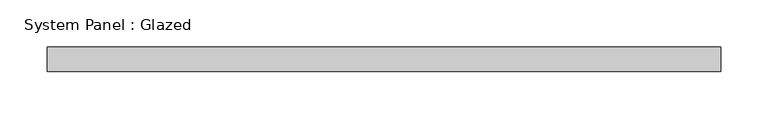
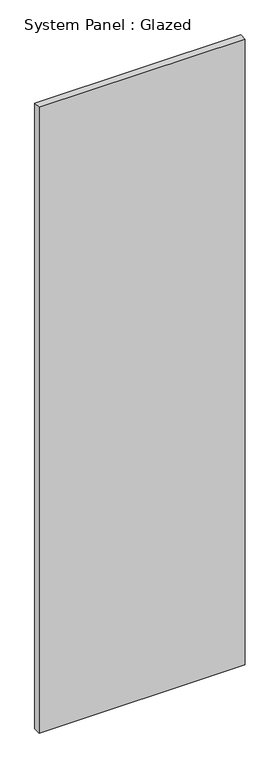
"""IFC4 building model written with IfcOpenShell, lengths in millimetres: plate geometry, System Panel : Glazed."""

from ifc_helpers import new_model, si_unit, origin, origin_with_axes, place, context, project, spatial, polyline, outline, extrude, source, transform, mapped, element, save


def system_panel_glazed_161bf594(model_context):
    return source(origin(), model_context, "Body", "SweptSolid", [
        extrude(outline(polyline([(354.5271, 19.05), (-354.5271, 19.05), (-354.5271, 44.45), (354.5271, 44.45), (354.5271, 19.05)])), origin_with_axes(), (0.0, 0.0, 1.0), 2275.4166667),
    ])


if __name__ == "__main__":
    model = new_model("IFC4")
    model_context = context("Model", 3, world=origin())
    ifc_project = project(units=[si_unit("LENGTHUNIT", "METRE", prefix="MILLI")], contexts=[model_context])
    site = spatial("IfcSite", under=ifc_project)
    building = spatial("IfcBuilding", under=site)
    placement = place(None, origin())
    system_panel_glazed_shape = system_panel_glazed_161bf594(model_context)
    element("IfcPlate", 1, ObjectType="System Panel : Glazed", at=placement, inside=building, context=model_context, shape_type="MappedRepresentation", body=[
        mapped(system_panel_glazed_shape, transform((0.0, 0.0, 0.0), x_axis=(1.0, 0.0, 0.0), y_axis=(0.0, 1.0, 0.0), z_axis=(0.0, 0.0, 1.0))),
    ])
    save(model, "model.ifc")

# Revit data of these elements
# Type "System Panel : Glazed"
#   Construction Type Id = "GSP4R"
#   Analytic Construction = "1/8 in Pilkington single glazing"
#   Visual Light Transmittance = 0.9
#   Solar Heat Gain Coefficient = 0.86
#   Heat Transfer Coefficient (U) = 1.18115 BTU/(h·ft²·°F)
#   Define Thermal Properties by = 1
# Element 1 (IfcPlate, "System Panel : Glazed")
#   Materials on its faces: "Glass"
# Materials
#   "Glass": class "Glass", colour RGB 0 128 192, transparency 0.75, Description = "Soda Lime Glass", Cost = 0
